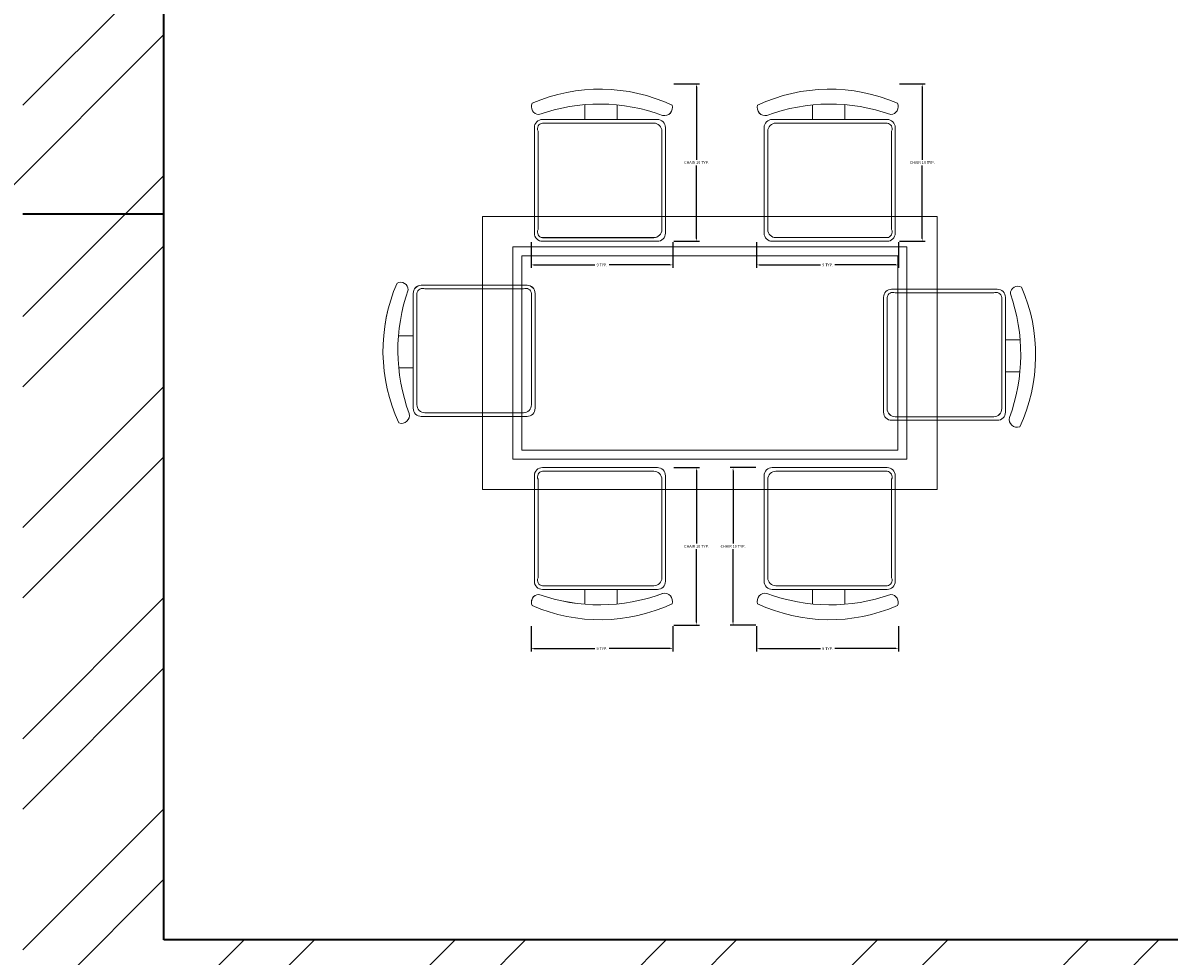
# Model space of a CAD drawing. Units: inches. Extents: x 2120 to 4013, y 1390 to 3019.
# Tile 19 of 59: x 2716 to 2789, y 1732 to 1792. Entities that reach past the tile are written whole.
import ezdxf

# ---------------------------------------------------------------- set-up
doc = ezdxf.new("R2010")
doc.units = ezdxf.units.IN
for name, color, linetype, lineweight in [('A-ANNO-DIMS', 2, 'Continuous', 18), ('A-FURN', 8, 'Continuous', 13), ('A-WALL', 7, 'Continuous', 35), ('A-WALL-PATT', 252, 'Continuous', 13)]:
    doc.layers.add(name, color=color, linetype=linetype, lineweight=lineweight)
doc.styles.get("Standard").update_dxf_attribs({"font": 'arial.ttf'})
doc.dimstyles.get("Standard").update_dxf_attribs({"dimtxt": 0.18, "dimasz": 0.18, "dimexe": 0.18, "dimexo": 0.0625, "dimgap": 0.09, "dimtad": 0, "dimtih": 1, "dimtoh": 1, "dimdec": 4, "dimzin": 0, "dimdsep": 46, "dimtxsty": 'Standard', "dimcen": 0.09, "dimadec": 0, "dimazin": 0, "dimtfac": 1, "dimtdec": 4, "dimtofl": 0, "dimtmove": 0, "dimatfit": 3, "dimfxl": 1, "dimtolj": 1, "dimtzin": 0, "dimarcsym": 0})

# ---------------------------------------------------------------- blocks, each defined once
blk = doc.blocks.new('TABLE-DINING')
for points in [[(0, 17.406), (29.011, 17.406), (29.011, 0), (0, 0)], [(1.934, 15.472), (27.077, 15.472), (27.077, 1.934), (1.934, 1.934)], [(2.514, 14.892), (26.496, 14.892), (26.496, 2.514), (2.514, 2.514)]]:
    blk.add_lwpolyline(points, close=True)
blk = doc.blocks.new('CHAIR-DINING-04')
for points in [[(7.771, 8.294, 0.414214), (7.258, 8.807), (0.513, 8.807, 0.414214), (0, 8.294), (0, 0.958, 0.414214), (0.513, 0.445), (7.258, 0.445, 0.414214), (7.771, 0.958), (7.771, 8.294)], [(8.089, 8.525, -0.175809), (8.029, 0.623, 0.578392), (8.687, 0.025, 0.214524), (8.807, 8.944, 0.552014), (8.089, 8.525, -0.065079)], [(7.771, 3.535), (8.699, 3.535, -0.064759)]]:
    blk.add_lwpolyline(points, format="xyb")
blk.add_lwpolyline([(7.54, 8.291), (7.54, 1.19, -0.414214), (7.027, 0.676), (0.744, 0.676, -0.414214), (0.231, 1.19), (0.231, 8.291, -0.512069), (0.744, 8.576), (7.027, 8.576, -0.512069)], format="xyb", close=True)
blk.add_lwpolyline([(8.716, 5.588), (7.771, 5.588)])
blk = doc.blocks.new('CHAIR-DINING-06')
for points in [[(7.771, 8.294, 0.414214), (7.258, 8.807), (0.513, 8.807, 0.414214), (0, 8.294), (0, 0.958, 0.414214), (0.513, 0.445), (7.258, 0.445, 0.414214), (7.771, 0.958), (7.771, 8.294)], [(8.089, 8.525, -0.175809), (8.029, 0.623, 0.578392), (8.687, 0.025, 0.214524), (8.807, 8.944, 0.552014), (8.089, 8.525, -0.065079)], [(7.771, 3.535), (8.699, 3.535, -0.064759)]]:
    blk.add_lwpolyline(points, format="xyb")
blk.add_lwpolyline([(7.54, 8.291), (7.54, 1.19, -0.414214), (7.027, 0.676), (0.744, 0.676, -0.414214), (0.231, 1.19), (0.231, 8.291, -0.512069), (0.744, 8.576), (7.027, 8.576, -0.512069)], format="xyb", close=True)
blk.add_lwpolyline([(8.716, 5.588), (7.771, 5.588)])
blk = doc.blocks.new('CHAIR-DINING-07')
for points in [[(0.623, 8.029, -0.578392), (0.025, 8.687, -0.214524), (8.944, 8.807, -0.552014), (8.525, 8.089, 0.175809), (0.623, 8.029)], [(3.535, 7.771), (3.535, 8.699, 0.064759)], [(8.294, 7.771, -0.414214), (8.807, 7.258), (8.807, 0.513, -0.414214), (8.294, 0), (0.958, 0, -0.414214), (0.445, 0.513), (0.445, 7.258, -0.414214), (0.958, 7.771), (8.294, 7.771)]]:
    blk.add_lwpolyline(points, format="xyb")
blk.add_lwpolyline([(5.588, 8.716), (5.588, 7.771)])
blk.add_lwpolyline([(8.291, 7.54), (1.19, 7.54, 0.414214), (0.676, 7.027), (0.676, 0.744, 0.414214), (1.19, 0.231), (8.291, 0.231, 0.512069), (8.576, 0.744), (8.576, 7.027, 0.512069)], format="xyb", close=True)
blk = doc.blocks.new('CHAIR-DINING-08')
for points in [[(0.475, 8.089, -0.175809), (8.376, 8.029, 0.578392), (8.975, 8.687, 0.214524), (0.056, 8.807, 0.552014), (0.475, 8.089, -0.065079)], [(5.464, 7.771), (5.464, 8.699, -0.064759)], [(8.041, 7.771), (0.705, 7.771, 0.414214), (0.192, 7.258), (0.192, 0.513, 0.414214), (0.705, 0), (8.041, 0, 0.414214), (8.554, 0.513), (8.554, 7.258, 0.414214), (8.041, 7.771)]]:
    blk.add_lwpolyline(points, format="xyb")
blk.add_lwpolyline([(3.411, 8.716), (3.411, 7.771)])
blk.add_lwpolyline([(0.709, 7.54), (7.81, 7.54, -0.414214), (8.323, 7.027), (8.323, 0.744, -0.414214), (7.81, 0.231), (0.709, 0.231, -0.512069), (0.423, 0.744), (0.423, 7.027, -0.512069)], format="xyb", close=True)
blk = doc.blocks.new('CHAIR-DINING-09')
for points in [[(0.475, 8.089, -0.175809), (8.376, 8.029, 0.578392), (8.975, 8.687, 0.214524), (0.056, 8.807, 0.552014), (0.475, 8.089, -0.065079)], [(5.464, 7.771), (5.464, 8.699, -0.064759)], [(8.041, 7.771), (0.705, 7.771, 0.414214), (0.192, 7.258), (0.192, 0.513, 0.414214), (0.705, 0), (8.041, 0, 0.414214), (8.554, 0.513), (8.554, 7.258, 0.414214), (8.041, 7.771)]]:
    blk.add_lwpolyline(points, format="xyb")
blk.add_lwpolyline([(3.411, 8.716), (3.411, 7.771)])
blk.add_lwpolyline([(0.709, 7.54), (7.81, 7.54, -0.414214), (8.323, 7.027), (8.323, 0.744, -0.414214), (7.81, 0.231), (0.709, 0.231, -0.512069), (0.423, 0.744), (0.423, 7.027, -0.512069)], format="xyb", close=True)
blk = doc.blocks.new('CHAIR-DINING-12')
for points in [[(7.771, 8.294, 0.414214), (7.258, 8.807), (0.513, 8.807, 0.414214), (0, 8.294), (0, 0.958, 0.414214), (0.513, 0.445), (7.258, 0.445, 0.414214), (7.771, 0.958), (7.771, 8.294)], [(8.089, 8.525, -0.175809), (8.029, 0.623, 0.578392), (8.687, 0.025, 0.214524), (8.807, 8.944, 0.552014), (8.089, 8.525, -0.065079)], [(7.771, 3.535), (8.699, 3.535, -0.064759)]]:
    blk.add_lwpolyline(points, format="xyb")
blk.add_lwpolyline([(7.54, 8.291), (7.54, 1.19, -0.414214), (7.027, 0.676), (0.744, 0.676, -0.414214), (0.231, 1.19), (0.231, 8.291, -0.512069), (0.744, 8.576), (7.027, 8.576, -0.512069)], format="xyb", close=True)
blk.add_lwpolyline([(8.716, 5.588), (7.771, 5.588)])
blk = doc.blocks.new('CHAIR-DINING-16')
for points in [[(8.041, 1.933), (0.705, 1.933, -0.414214), (0.192, 2.446), (0.192, 9.191, -0.414214), (0.705, 9.704), (8.041, 9.704, -0.414214), (8.554, 9.191), (8.554, 2.446, -0.414214), (8.041, 1.933)], [(8.376, 1.676, -0.578392), (8.975, 1.018, -0.214524), (0.056, 0.898, -0.552014), (0.475, 1.616, 0.175809), (8.376, 1.676)], [(5.464, 1.933), (5.464, 1.005, 0.064759)]]:
    blk.add_lwpolyline(points, format="xyb")
blk.add_lwpolyline([(0.709, 2.164), (7.81, 2.164, 0.414214), (8.323, 2.677), (8.323, 8.96, 0.414214), (7.81, 9.473), (0.709, 9.473, 0.512069), (0.423, 8.96), (0.423, 2.677, 0.512069)], format="xyb", close=True)
blk.add_lwpolyline([(3.411, 0.988), (3.411, 1.933)])
blk = doc.blocks.new('*D87')
at = {"layer": 'A-ANNO-DIMS', "color": 0, "lineweight": -2, "transparency": 16777216}
for p, q in [((2762.484, 1763.158), (2760.86, 1763.158)), ((2761.04, 1762.978), (2761.04, 1758.319)), ((2761.04, 1753.294), (2761.04, 1757.953)), ((2762.484, 1753.114), (2760.86, 1753.114))]:
    blk.add_line(p, q, dxfattribs=at)
at = {"layer": 'A-ANNO-DIMS', "color": 0, "transparency": 16777216}
for points in [[(2761.01, 1762.978), (2761.07, 1762.978), (2761.04, 1763.158)], [(2761.01, 1753.294), (2761.07, 1753.294), (2761.04, 1753.114)]]:
    blk.add_solid(points, dxfattribs=at)
at = {"layer": 'Defpoints', "color": 0, "transparency": 16777216}
for p in [(2762.546, 1763.158), (2761.04, 1753.114), (2762.546, 1753.114)]:
    blk.add_point(p, dxfattribs=at)
at = {"layer": 'A-ANNO-DIMS', "color": 0, "transparency": 16777216, "insert": (2761.04, 1758.136), "char_height": 0.18, "attachment_point": 5}
blk.add_mtext('\\A1;CHAIR 10 TYP.', dxfattribs=at)
blk = doc.blocks.new('*D88')
at = {"layer": 'A-ANNO-DIMS', "color": 0, "lineweight": -2, "transparency": 16777216}
for p, q in [((2762.546, 1753.052), (2762.546, 1751.428)), ((2771.6, 1753.052), (2771.6, 1751.428)), ((2762.726, 1751.608), (2766.615, 1751.608)), ((2771.42, 1751.608), (2767.531, 1751.608))]:
    blk.add_line(p, q, dxfattribs=at)
at = {"layer": 'A-ANNO-DIMS', "color": 0, "transparency": 16777216}
for points in [[(2762.726, 1751.638), (2762.726, 1751.578), (2762.546, 1751.608)], [(2771.42, 1751.638), (2771.42, 1751.578), (2771.6, 1751.608)]]:
    blk.add_solid(points, dxfattribs=at)
at = {"layer": 'Defpoints', "color": 0, "transparency": 16777216}
for p in [(2762.546, 1753.114), (2771.6, 1753.114), (2771.6, 1751.608)]:
    blk.add_point(p, dxfattribs=at)
at = {"layer": 'A-ANNO-DIMS', "color": 0, "transparency": 16777216, "insert": (2767.073, 1751.608), "char_height": 0.18, "attachment_point": 5}
blk.add_mtext('\\A1;9 TYP.', dxfattribs=at)
blk = doc.blocks.new('*D93')
at = {"layer": 'A-ANNO-DIMS', "color": 0, "lineweight": -2, "transparency": 16777216}
for p, q in [((2771.662, 1787.643), (2773.287, 1787.643)), ((2773.107, 1787.463), (2773.107, 1782.804)), ((2773.107, 1777.779), (2773.107, 1782.438)), ((2771.662, 1777.599), (2773.287, 1777.599))]:
    blk.add_line(p, q, dxfattribs=at)
at = {"layer": 'A-ANNO-DIMS', "color": 0, "transparency": 16777216}
for points in [[(2773.077, 1787.463), (2773.137, 1787.463), (2773.107, 1787.643)], [(2773.077, 1777.779), (2773.137, 1777.779), (2773.107, 1777.599)]]:
    blk.add_solid(points, dxfattribs=at)
at = {"layer": 'Defpoints', "color": 0, "transparency": 16777216}
for p in [(2771.6, 1787.643), (2773.107, 1787.643), (2771.6, 1777.599)]:
    blk.add_point(p, dxfattribs=at)
at = {"layer": 'A-ANNO-DIMS', "color": 0, "transparency": 16777216, "insert": (2773.107, 1782.621), "char_height": 0.18, "attachment_point": 5}
blk.add_mtext('\\A1;CHAIR 10 TYP.', dxfattribs=at)
blk = doc.blocks.new('*D94')
at = {"layer": 'A-ANNO-DIMS', "color": 0, "lineweight": -2, "transparency": 16777216}
for p, q in [((2762.546, 1777.537), (2762.546, 1775.912)), ((2771.6, 1777.537), (2771.6, 1775.912)), ((2762.726, 1776.092), (2766.615, 1776.092)), ((2771.42, 1776.092), (2767.531, 1776.092))]:
    blk.add_line(p, q, dxfattribs=at)
at = {"layer": 'A-ANNO-DIMS', "color": 0, "transparency": 16777216}
for points in [[(2762.726, 1776.122), (2762.726, 1776.062), (2762.546, 1776.092)], [(2771.42, 1776.122), (2771.42, 1776.062), (2771.6, 1776.092)]]:
    blk.add_solid(points, dxfattribs=at)
at = {"layer": 'Defpoints', "color": 0, "transparency": 16777216}
for p in [(2762.546, 1777.599), (2771.6, 1777.599), (2771.6, 1776.092)]:
    blk.add_point(p, dxfattribs=at)
at = {"layer": 'A-ANNO-DIMS', "color": 0, "transparency": 16777216, "insert": (2767.073, 1776.092), "char_height": 0.18, "attachment_point": 5}
blk.add_mtext('\\A1;9 TYP.', dxfattribs=at)
blk = doc.blocks.new('*D95')
at = {"layer": 'A-ANNO-DIMS', "color": 0, "lineweight": -2, "transparency": 16777216}
for p, q in [((2757.266, 1787.643), (2758.89, 1787.643)), ((2758.71, 1787.463), (2758.71, 1782.804)), ((2758.71, 1777.779), (2758.71, 1782.438)), ((2757.266, 1777.599), (2758.89, 1777.599))]:
    blk.add_line(p, q, dxfattribs=at)
at = {"layer": 'A-ANNO-DIMS', "color": 0, "transparency": 16777216}
for points in [[(2758.68, 1787.463), (2758.74, 1787.463), (2758.71, 1787.643)], [(2758.68, 1777.779), (2758.74, 1777.779), (2758.71, 1777.599)]]:
    blk.add_solid(points, dxfattribs=at)
at = {"layer": 'Defpoints', "color": 0, "transparency": 16777216}
for p in [(2757.204, 1787.643), (2758.71, 1787.643), (2757.204, 1777.599)]:
    blk.add_point(p, dxfattribs=at)
at = {"layer": 'A-ANNO-DIMS', "color": 0, "transparency": 16777216, "insert": (2758.71, 1782.621), "char_height": 0.18, "attachment_point": 5}
blk.add_mtext('\\A1;CHAIR 10 TYP.', dxfattribs=at)
blk = doc.blocks.new('*D96')
at = {"layer": 'A-ANNO-DIMS', "color": 0, "lineweight": -2, "transparency": 16777216}
for p, q in [((2748.15, 1777.536), (2748.15, 1775.912)), ((2757.204, 1777.536), (2757.204, 1775.912)), ((2748.33, 1776.092), (2752.219, 1776.092)), ((2757.024, 1776.092), (2753.135, 1776.092))]:
    blk.add_line(p, q, dxfattribs=at)
at = {"layer": 'A-ANNO-DIMS', "color": 0, "transparency": 16777216}
for points in [[(2748.33, 1776.122), (2748.33, 1776.062), (2748.15, 1776.092)], [(2757.024, 1776.122), (2757.024, 1776.062), (2757.204, 1776.092)]]:
    blk.add_solid(points, dxfattribs=at)
at = {"layer": 'Defpoints', "color": 0, "transparency": 16777216}
for p in [(2748.15, 1777.599), (2757.204, 1777.599), (2757.204, 1776.092)]:
    blk.add_point(p, dxfattribs=at)
at = {"layer": 'A-ANNO-DIMS', "color": 0, "transparency": 16777216, "insert": (2752.677, 1776.092), "char_height": 0.18, "attachment_point": 5}
blk.add_mtext('\\A1;9 TYP.', dxfattribs=at)
blk = doc.blocks.new('*D111')
at = {"layer": 'A-ANNO-DIMS', "color": 0, "lineweight": -2, "transparency": 16777216}
for p, q in [((2757.266, 1763.159), (2758.89, 1763.159)), ((2758.71, 1762.979), (2758.71, 1758.32)), ((2758.71, 1753.295), (2758.71, 1757.954)), ((2757.266, 1753.115), (2758.89, 1753.115))]:
    blk.add_line(p, q, dxfattribs=at)
at = {"layer": 'A-ANNO-DIMS', "color": 0, "transparency": 16777216}
for points in [[(2758.68, 1762.979), (2758.74, 1762.979), (2758.71, 1763.159)], [(2758.68, 1753.295), (2758.74, 1753.295), (2758.71, 1753.115)]]:
    blk.add_solid(points, dxfattribs=at)
at = {"layer": 'Defpoints', "color": 0, "transparency": 16777216}
for p in [(2757.204, 1763.159), (2758.71, 1763.159), (2757.204, 1753.115)]:
    blk.add_point(p, dxfattribs=at)
at = {"layer": 'A-ANNO-DIMS', "color": 0, "transparency": 16777216, "insert": (2758.71, 1758.137), "char_height": 0.18, "attachment_point": 5}
blk.add_mtext('\\A1;CHAIR 10 TYP.', dxfattribs=at)
blk = doc.blocks.new('*D112')
at = {"layer": 'A-ANNO-DIMS', "color": 0, "lineweight": -2, "transparency": 16777216}
for p, q in [((2748.15, 1753.052), (2748.15, 1751.428)), ((2757.204, 1753.052), (2757.204, 1751.428)), ((2748.33, 1751.608), (2752.219, 1751.608)), ((2757.024, 1751.608), (2753.135, 1751.608))]:
    blk.add_line(p, q, dxfattribs=at)
at = {"layer": 'A-ANNO-DIMS', "color": 0, "transparency": 16777216}
for points in [[(2748.33, 1751.638), (2748.33, 1751.578), (2748.15, 1751.608)], [(2757.024, 1751.638), (2757.024, 1751.578), (2757.204, 1751.608)]]:
    blk.add_solid(points, dxfattribs=at)
at = {"layer": 'Defpoints', "color": 0, "transparency": 16777216}
for p in [(2748.15, 1753.115), (2757.204, 1753.115), (2757.204, 1751.608)]:
    blk.add_point(p, dxfattribs=at)
at = {"layer": 'A-ANNO-DIMS', "color": 0, "transparency": 16777216, "insert": (2752.677, 1751.608), "char_height": 0.18, "attachment_point": 5}
blk.add_mtext('\\A1;9 TYP.', dxfattribs=at)

msp = doc.modelspace()

# ---------------------------------------------------------------- hatches: boundary and pattern name
at = {"layer": 'A-WALL-PATT'}
h = msp.add_hatch(dxfattribs=at)
h.set_pattern_fill('ANSI32', color=256)
h.paths.add_polyline_path([(2271.7331, 2122.6377), (2262.7331, 2122.6377), (2262.7331, 2040.3893), (2267.2331, 2040.3893), (2271.7331, 2040.3893), (2271.7331, 2044.8856), (2271.7331, 2070.531), (2391.7331, 2070.531), (2391.7331, 1926.5306), (2388.3993, 1926.5306), (2388.3993, 1922.531), (2395.7331, 1922.531), (2395.7331, 1992.531), (2400.4511, 1992.531), (2400.4511, 1997.0306), (2395.7331, 1997.0306), (2395.7331, 2070.531), (2443.7331, 2070.531), (2443.7331, 2046.1368), (2448.2331, 2046.1368), (2448.2331, 2070.531), (2580.2331, 2070.531), (2580.2331, 1997.0306), (2492.9076, 1997.0306), (2492.9076, 1992.531), (2580.2331, 1992.531), (2580.2331, 1983.9368), (2589.2331, 1983.9368), (2589.2331, 2070.531), (2589.2331, 2075.0306), (2396.2331, 2075.0306), (2396.2331, 2184.3565), (2393.9831, 2184.3565), (2391.7331, 2184.3565), (2391.7331, 2075.0306), (2271.7331, 2075.0306)])
h.paths.add_polyline_path([(2724.7331, 2138.0306), (2628.7331, 2138.0306), (2628.7331, 2070.5306), (2628.7331, 2067.0987), (2633.2331, 2067.0987), (2637.7331, 2067.0987), (2637.7331, 2070.531), (2657.3413, 2070.531), (2657.3413, 2079.5306), (2637.7331, 2079.5306), (2637.7331, 2129.031), (2715.7331, 2129.031), (2715.7331, 2079.5306), (2698.0378, 2079.5306), (2698.0378, 2070.531), (2715.7331, 2070.531), (2715.7331, 2012.1531), (2720.2331, 2012.1531), (2724.7331, 2012.1531)])
h.paths.add_polyline_path([(2724.7331, 2213.031), (2831.3209, 2213.031), (2831.3209, 2215.281), (2831.3209, 2217.5306), (2724.7331, 2217.5306), (2724.7331, 2343.531), (2751.8755, 2343.531), (2751.8755, 2352.5306), (2715.7331, 2352.5306), (2715.7331, 2138.031), (2724.7331, 2138.031)])
h.paths.add_polyline_path([(2902.53, 2352.5306), (2811.8755, 2352.5306), (2811.8755, 2343.531), (2867.2331, 2343.531), (2867.2331, 2217.5306), (2863.6364, 2217.5306), (2863.6364, 2213.031), (2871.7331, 2213.031), (2871.7331, 2217.531), (2871.7331, 2343.531), (2902.53, 2343.531)])
h.paths.add_polyline_path([(3009.7331, 2352.5306), (2938.53, 2352.5306), (2938.53, 2343.531), (2966.2331, 2343.531), (2966.2331, 2242.3281), (2968.4831, 2242.3281), (2970.7331, 2242.3281), (2970.7331, 2343.531), (3009.7331, 2343.531)])
h.paths.add_polyline_path([(3009.7331, 2217.5306), (2970.7331, 2217.5306), (2970.7331, 2220.5422), (2968.4831, 2220.5422), (2966.2331, 2220.5422), (2966.2331, 2217.5306), (2911.7752, 2217.5306), (2907.7331, 2217.5306), (2907.7331, 2213.0306), (2907.7331, 2194.9663), (2912.2331, 2194.9663), (2912.2331, 2213.031), (2970.7331, 2213.031), (3000.7331, 2213.031), (3000.7331, 2205.523), (3009.7331, 2205.523)])
h.paths.add_polyline_path([(3009.7331, 2181.5227), (3000.7331, 2181.5227), (3000.7331, 2165.0306), (2912.2331, 2165.0306), (2912.2331, 2170.8202), (2907.7331, 2170.8202), (2907.7331, 2165.0306), (2899.5169, 2165.0306), (2899.5169, 2162.7806), (2899.5169, 2160.531), (2907.7331, 2160.531), (2907.7331, 2137.3432), (2912.2331, 2137.3432), (2912.2331, 2160.531), (3000.7331, 2160.531), (3000.7331, 2150.4993), (3009.7331, 2150.4993)])
h.paths.add_polyline_path([(3009.7331, 2126.499), (3005.2331, 2126.499), (3000.7331, 2126.499), (3000.7331, 2112.5306), (2912.2331, 2112.5306), (2912.2331, 2115.6036), (2907.7331, 2115.6036), (2907.7331, 2108.031), (3000.7331, 2108.031), (3000.7331, 2084.7256), (3009.7331, 2084.7256)], flags=17)
h.paths.add_polyline_path([(3009.7331, 1971.531), (3009.7331, 2024.7253), (3000.7331, 2024.7253), (3000.7331, 2006.4153), (3000.7331, 1971.5306), (2864.2331, 1971.5306), (2864.2331, 2160.531), (2868.0522, 2160.531), (2868.0522, 2165.0306), (2859.7331, 2165.0306), (2859.7331, 1971.5306), (2724.7331, 1971.5306), (2724.7331, 1977.7012), (2715.7331, 1977.7012), (2715.7331, 1962.5306), (2715.7331, 1950.9035), (2720.2331, 1950.9035), (2724.7331, 1950.9035), (2724.7331, 1962.531), (2855.2331, 1962.531), (2859.7331, 1962.531), (2859.7331, 1835.031), (2864.2331, 1834.8158), (2864.2331, 1962.531), (2958.7331, 1962.531), (2958.7331, 1937.0925), (2963.2331, 1937.0925), (2963.2331, 1962.531), (3000.7331, 1962.531), (3009.7331, 1962.531)])
h.paths.add_polyline_path([(2724.7331, 1728.531), (2822.7164, 1728.531), (2822.7164, 1733.0306), (2724.7331, 1733.0306), (2724.7331, 1779.3416), (2715.7331, 1779.3416), (2715.7331, 1581.531), (2753.02, 1581.531), (2753.02, 1586.031), (2753.02, 1590.5306), (2724.7331, 1590.5306)])
h.paths.add_polyline_path([(2864.2331, 1590.531), (2864.2331, 1787.031), (2868.4075, 1787.031), (2868.4075, 1791.5306), (2859.7331, 1791.5306), (2859.7331, 1739.0306), (2859.7331, 1733.0306), (2854.3125, 1733.0306), (2854.3125, 1728.531), (2859.7331, 1728.531), (2859.7331, 1590.5306), (2813.02, 1590.5306), (2813.02, 1581.531), (2868.4123, 1581.531), (2868.4123, 1583.781), (2868.4123, 1586.0306), (2864.2331, 1586.0306)])
h.paths.add_polyline_path([(3009.7331, 1754.6619), (3000.7331, 1754.6619), (3000.7331, 1739.0306), (2912.2331, 1739.0306), (2912.2331, 1742.2257), (2907.7331, 1742.2257), (2907.7331, 1739.0306), (2907.7331, 1734.531), (3000.7331, 1734.531), (3000.7331, 1590.5306), (3000.7331, 1586.0306), (2971.3921, 1586.0306), (2971.3921, 1581.531), (3009.7331, 1581.531)])
h.paths.add_polyline_path([(2911.3921, 1583.781), (2911.3921, 1586.0306), (2891.2138, 1586.0306), (2891.2138, 1581.531), (2911.3921, 1581.531)])
h.paths.add_polyline_path([(3009.7331, 1799.8422), (3000.7331, 1799.8422), (3000.7331, 1791.5306), (2912.2331, 1791.5306), (2912.2331, 1796.3264), (2909.9831, 1796.3264), (2907.7331, 1796.3264), (2907.7331, 1791.5306), (2902.7033, 1791.5306), (2902.7033, 1787.031), (2907.7331, 1787.031), (2907.7331, 1761.1622), (2912.2331, 1761.1622), (2912.2331, 1787.031), (3000.7331, 1787.031), (3000.7331, 1778.6622), (3009.7331, 1778.6622)])
h.paths.add_polyline_path([(3009.7331, 1839.5306), (2963.2331, 1839.5306), (2963.2331, 1842.8629), (2960.9831, 1842.8629), (2958.7331, 1842.8629), (2958.7331, 1839.5306), (2907.7331, 1839.5306), (2907.7331, 1814.4599), (2912.2331, 1814.4599), (2912.2331, 1835.031), (3000.7331, 1835.031), (3000.7331, 1823.8425), (3009.7331, 1823.8425), (3009.7331, 1835.031)])
h.paths.add_polyline_path([(2963.2331, 1901.0922), (2960.9831, 1901.0922), (2958.7331, 1901.0922), (2958.7331, 1862.8843), (2963.2331, 1862.8843)], flags=17)
h.paths.add_polyline_path([(2724.7331, 1891.9826), (2724.7331, 1914.3416), (2715.7331, 1914.3416), (2715.7331, 1783.8416), (2637.7331, 1783.8416), (2637.7331, 1914.3416), (2628.7331, 1914.3416), (2624.7701, 1914.3416), (2624.7701, 1909.8416), (2624.7701, 1905.3419), (2628.7331, 1905.3419), (2628.7331, 1876.9915), (2628.7331, 1779.3419), (2637.7331, 1779.3419), (2715.7331, 1779.3419), (2724.7331, 1779.3419), (2724.7331, 1835.031)])
h.paths.add_polyline_path([(2637.7331, 1731.531), (2637.7331, 1779.3416), (2628.7331, 1779.3416), (2628.7331, 1731.5306), (2589.2331, 1731.5306), (2535.9814, 1731.5306), (2496.7331, 1731.5306), (2496.7331, 1725.6876), (2498.9831, 1725.6876), (2501.2331, 1725.6876), (2501.2331, 1727.031), (2628.7331, 1727.031), (2628.7331, 1680.4203), (2628.7331, 1590.5306), (2628.7331, 1586.0306), (2604.1361, 1586.0306), (2604.1361, 1581.531), (2637.7331, 1581.531), (2637.7331, 1590.531)])

# ---------------------------------------------------------------- linework, layer by layer
at = {"layer": 'A-FURN'}
for points in [[(2763.2012, 1785.6275, -0.5783921), (2762.6026, 1786.2857, -0.2145244), (2771.5219, 1786.4054, -0.552014), (2771.1029, 1785.6873, 0.1758092), (2763.2012, 1785.6275)], [(2766.1131, 1785.3702), (2766.1131, 1786.2979, 0.0647586)], [(2770.8721, 1785.3702, -0.4142136), (2771.3853, 1784.857), (2771.3853, 1778.112, -0.4142136), (2770.8721, 1777.5988), (2763.5364, 1777.5988, -0.4142136), (2763.0232, 1778.112), (2763.0232, 1784.857, -0.4142136), (2763.5364, 1785.3702), (2770.8721, 1785.3702)], [(2740.3806, 1766.6062, -0.5783921), (2739.7224, 1766.0076, -0.2145244), (2739.6027, 1774.927, -0.552014), (2740.3207, 1774.5079, 0.1758094), (2740.3806, 1766.6062)], [(2740.6379, 1774.2771, -0.4142136), (2741.1511, 1774.7904), (2747.8961, 1774.7904, -0.4142136), (2748.4093, 1774.2771), (2748.4093, 1766.9415, -0.4142136), (2747.8961, 1766.4283), (2741.1511, 1766.4283, -0.4142136), (2740.6379, 1766.9415), (2740.6379, 1774.2771)], [(2740.6379, 1769.5181), (2739.7101, 1769.5181, 0.0647586)], [(2756.2138, 1755.387), (2748.8781, 1755.387, -0.4142136), (2748.3649, 1755.9002), (2748.3649, 1762.6452, -0.4142136), (2748.8781, 1763.1584), (2756.2138, 1763.1584, -0.4142136), (2756.727, 1762.6452), (2756.727, 1755.9002, -0.4142136), (2756.2138, 1755.387)], [(2756.549, 1755.1297, -0.5783921), (2757.1476, 1754.4715, -0.2145244), (2748.2283, 1754.3518, -0.552014), (2748.6473, 1755.0698, 0.1758093), (2756.549, 1755.1297)], [(2753.6371, 1755.387), (2753.6371, 1754.4592, 0.0647586)]]:
    msp.add_lwpolyline(points, format="xyb", dxfattribs=at)
for points in [[(2768.1665, 1786.3148), (2768.1665, 1785.3702)], [(2739.6933, 1771.5715), (2740.6379, 1771.5715)], [(2751.5837, 1754.4424), (2751.5837, 1755.387)]]:
    msp.add_lwpolyline(points, dxfattribs=at)
for points in [[(2770.869, 1785.139), (2763.7677, 1785.139, 0.4142136), (2763.2544, 1784.6258), (2763.2544, 1778.3432, 0.4142136), (2763.7677, 1777.83), (2770.869, 1777.83, 0.5120695), (2771.1541, 1778.3432), (2771.1541, 1784.6258, 0.5120695)], [(2740.8691, 1774.274), (2740.8691, 1767.1727, 0.4142136), (2741.3823, 1766.6595), (2747.6649, 1766.6595, 0.4142136), (2748.1781, 1767.1727), (2748.1781, 1774.274, 0.5120695), (2747.6649, 1774.5592), (2741.3823, 1774.5592, 0.5120695)], [(2748.8812, 1755.6182), (2755.9826, 1755.6182, 0.4142136), (2756.4958, 1756.1314), (2756.4958, 1762.414, 0.4142136), (2755.9826, 1762.9272), (2748.8812, 1762.9272, 0.5120695), (2748.5961, 1762.414), (2748.5961, 1756.1314, 0.5120695)]]:
    msp.add_lwpolyline(points, format="xyb", close=True, dxfattribs=at)
at = {"layer": 'A-WALL'}
for p, q in [((2724.7331, 1733.031), (2724.7331, 1835.031)), ((2724.7331, 1733.0306), (2724.7331, 1835.0306)), ((2715.7331, 1779.3419), (2724.7331, 1779.3419)), ((2715.7331, 1779.3416), (2724.7331, 1779.3416)), ((2822.7164, 1733.031), (2724.7331, 1733.031)), ((2822.7164, 1733.0306), (2724.7331, 1733.0306))]:
    msp.add_line(p, q, dxfattribs=at)

# ---------------------------------------------------------------- block references
at = {"layer": 'A-FURN'}
for name, p in [('CHAIR-DINING-09', (2748.1726, 1777.5991)), ('CHAIR-DINING-08', (2748.1726, 1777.5988)), ('CHAIR-DINING-07', (2762.578, 1777.5991)), ('TABLE-DINING', (2745.0589, 1761.7689)), ('TABLE-DINING', (2745.059, 1761.7686)), ('CHAIR-DINING-06', (2770.6417, 1765.7318)), ('CHAIR-DINING-12', (2770.6417, 1765.7315)), ('CHAIR-DINING-16', (2748.1726, 1753.4542))]:
    msp.add_blockref(name, p, dxfattribs=at)
for name, p, rotation in [('CHAIR-DINING-07', (2748.4093, 1765.9827), 90.00000190782868), ('CHAIR-DINING-06', (2762.578, 1763.1587), 270.0000009021327), ('CHAIR-DINING-04', (2762.578, 1763.1584), 270.0000009021437)]:
    msp.add_blockref(name, p, dxfattribs=dict(at, rotation=rotation))

# ---------------------------------------------------------------- dimensions: what is measured, and where the dimension line sits
at = {"layer": 'A-ANNO-DIMS'}
for base, p1, p2, angle, text, picture, middle in [((2758.7104, 1787.643), (2757.2038, 1777.5988), (2757.2038, 1787.643), 90, 'CHAIR <> TYP.', '*D95', (2758.7104, 1782.6209)), ((2773.1066, 1787.6433), (2771.5999, 1777.5991), (2771.5999, 1787.6433), 90, 'CHAIR <> TYP.', '*D93', (2773.1066, 1782.6212)), ((2758.7104, 1763.1587), (2757.2037, 1753.1145), (2757.2037, 1763.1587), 90, 'CHAIR <> TYP.', '*D111', (2758.7104, 1758.1366)), ((2761.0398, 1753.1142), (2762.5464, 1763.1584), (2762.5464, 1753.1142), 270.000001, 'CHAIR <> TYP.', '*D87', (2761.0398, 1758.1363)), ((2771.6, 1751.6076), (2762.5464, 1753.1142), (2771.6, 1753.1142), 0.000001, '<> TYP.', '*D88', (2767.0732, 1751.6076))]:
    dim = msp.add_linear_dim(base=base, p1=p1, p2=p2, angle=angle, text=text, dimstyle='Standard', override={"dimdec": 0, "dimlfac": 1, "dimrnd": 0, "dimzin": 0, "dimdsep": 46, "dimlunit": 2}, dxfattribs=at)
    dim.commit()
    dim.dimension.update_dxf_attribs({"geometry": picture, "text_midpoint": middle})
for base, p1, p2, picture, middle in [((2757.2038, 1776.0921), (2748.1502, 1777.5988), (2757.2038, 1777.5988), '*D96', (2752.677, 1776.0921)), ((2771.5999, 1776.0924), (2762.5464, 1777.5991), (2771.5999, 1777.5991), '*D94', (2767.0732, 1776.0924)), ((2757.2037, 1751.6079), (2748.1502, 1753.1145), (2757.2037, 1753.1145), '*D112', (2752.677, 1751.6079))]:
    dim = msp.add_linear_dim(base=base, p1=p1, p2=p2, text='<> TYP.', dimstyle='Standard', override={"dimdec": 0, "dimlfac": 1, "dimrnd": 0, "dimzin": 0, "dimdsep": 46, "dimlunit": 2}, dxfattribs=at)
    dim.commit()
    dim.dimension.update_dxf_attribs({"geometry": picture, "text_midpoint": middle})

doc.saveas('drawing.dxf')
